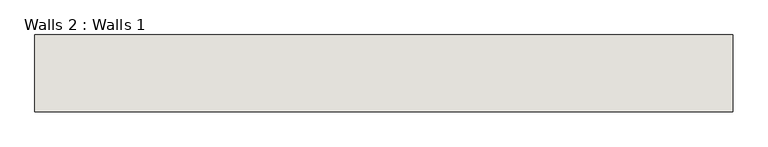
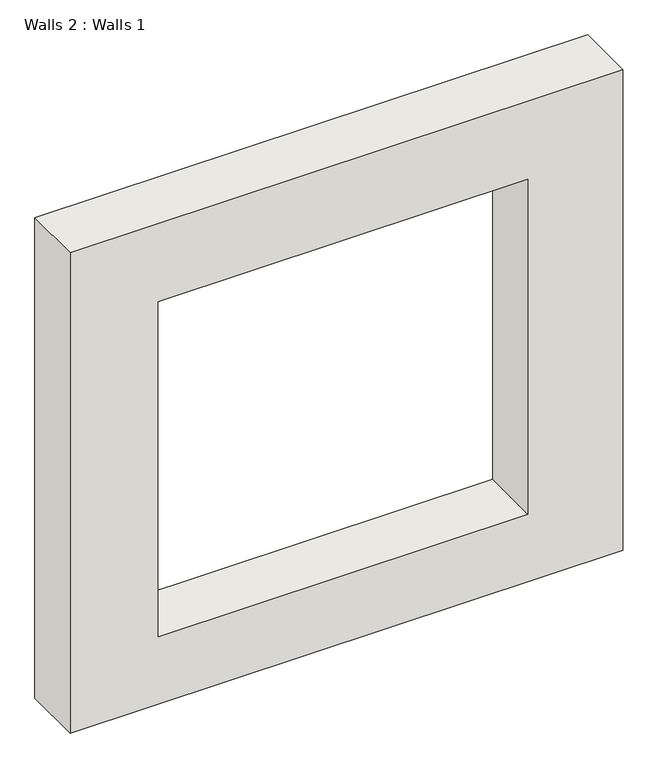
"""IFC4 building model written with IfcOpenShell, lengths in millimetres: wall geometry, Walls 2 : Walls 1."""

from ifc_helpers import new_model, si_unit, frame, origin, place, context, project, spatial, polyline, outline, extrude, source, transform, mapped, element, save


def walls_2_walls_1_3adabfa7(model_context):
    return source(origin(), model_context, "Body", "SweptSolid", [
        extrude(outline(polyline([(14297.1789316, -6069.6817469), (14297.1789316, -8558.8817469), (12011.1789316, -8558.8817469), (12011.1789316, -6069.6817469), (14297.1789316, -6069.6817469)]), holes=[polyline([(13925.6681256, -6498.1357575), (12331.8181256, -6498.1357575), (12331.8181256, -8161.8357575), (13925.6681256, -8161.8357575), (13925.6681256, -6498.1357575)])]), frame((0.0, 1408.0209854, 0.0), z_axis=(0.0, 1.0, 0.0), x_axis=(0.0, 0.0, 1.0)), (0.0, 0.0, 1.0), 274.2274628),
    ])


if __name__ == "__main__":
    model = new_model("IFC4")
    model_context = context("Model", 3, world=origin())
    ifc_project = project(units=[si_unit("LENGTHUNIT", "METRE", prefix="MILLI")], contexts=[model_context])
    site = spatial("IfcSite", under=ifc_project)
    building = spatial("IfcBuilding", under=site)
    placement = place(None, origin())
    walls_2_walls_1_shape = walls_2_walls_1_3adabfa7(model_context)
    element("IfcWall", 1, ObjectType="Walls 2 : Walls 1", at=placement, inside=building, context=model_context, shape_type="MappedRepresentation", body=[
        mapped(walls_2_walls_1_shape, transform((0.0, 0.0, 0.0), x_axis=(1.0, 0.0, 0.0), y_axis=(0.0, 1.0, 0.0), z_axis=(0.0, 0.0, 1.0))),
    ])
    save(model, "model.ifc")

# Revit data of these elements
# Element 1 (IfcWall, "Walls 2 : Walls 1")
#   Materials on its faces: "Default Wall"
# Materials
#   "Default Wall": colour RGB 128 128 128, transparency 0
